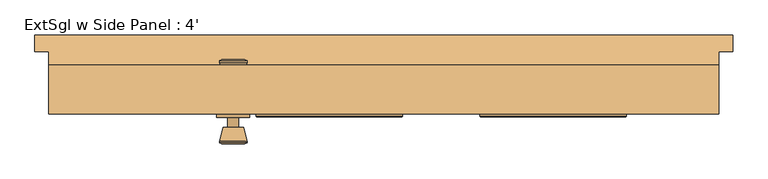
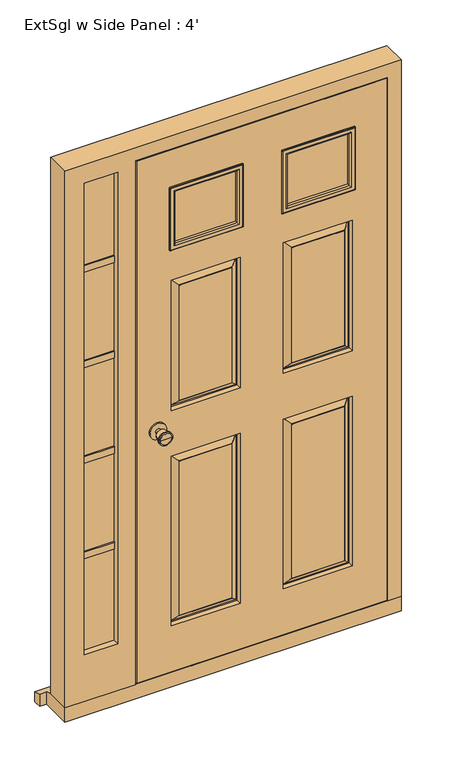
"""IFC4 building model written with IfcOpenShell, lengths in millimetres: door geometry, ExtSgl w Side Panel : 4'."""

from ifc_helpers import new_model, si_unit, point, frame, frame_2d, origin, place, context, project, spatial, polyline, circle_curve, ellipse_curve, trimmed, segment, composite_curve, outline, extrude, faceted_brep, source, transform, mapped, element, save
from ifc_brep_helpers import plane_surface, cylinder_surface, revolved_surface, advanced_brep


def extsgl_w_side_panel_4_ddded634(model_context):
    return source(origin(), model_context, "Body", "SolidModel", [
        advanced_brep(
        [(-493.3, -5.7, 1000.0), (-483.3, -5.7, 1000.0), (-503.3, -5.7, 1000.0), (-472.8241324, -54.7, 1000.0), (-493.3, -54.7, 1000.0), (-513.7758676, -54.7, 1000.0), (-468.3, -52.8721319, 1000.0), (-518.3, -52.8721319, 1000.0), (-468.3, -49.4084537, 1000.0), (-518.3, -49.4084537, 1000.0), (-474.663764, -24.7, 1000.0), (-511.936236, -24.7, 1000.0), (-483.3, -24.7, 1000.0), (-503.3, -24.7, 1000.0)],
        [
            (0, 1),
            (1, 2, circle_curve(frame((-493.3, -5.7, 1000.0), z_axis=(0.0, 1.0, 0.0), x_axis=(-1.0, 0.0, 0.0)), 10.0)),
            (2, 0),
            (2, 1, circle_curve(frame((-493.3, -5.7, 1000.0), z_axis=(0.0, 1.0, 0.0), x_axis=(-1.0, 0.0, 0.0)), 10.0)),
            (3, 4),
            (4, 5),
            (5, 3, circle_curve(frame((-493.3, -54.7, 1000.0), z_axis=(0.0, -1.0, 0.0), x_axis=(-1.0, 0.0, 0.0)), 20.4758676)),
            (3, 5, circle_curve(frame((-493.3, -54.7, 1000.0), z_axis=(0.0, -1.0, 0.0), x_axis=(-1.0, 0.0, 0.0)), 20.4758676)),
            (6, 3),
            (5, 7),
            (7, 6, circle_curve(frame((-493.3, -52.8721319, 1000.0), z_axis=(0.0, -1.0, 0.0), x_axis=(-1.0, 0.0, 0.0)), 25.0)),
            (6, 7, circle_curve(frame((-493.3, -52.8721319, 1000.0), z_axis=(0.0, -1.0, 0.0), x_axis=(-1.0, 0.0, 0.0)), 25.0)),
            (8, 6),
            (7, 9),
            (9, 8, circle_curve(frame((-493.3, -49.4084537, 1000.0), z_axis=(0.0, -1.0, 0.0), x_axis=(-1.0, 0.0, 0.0)), 25.0)),
            (8, 9, circle_curve(frame((-493.3, -49.4084537, 1000.0), z_axis=(0.0, -1.0, 0.0), x_axis=(-1.0, 0.0, 0.0)), 25.0)),
            (10, 8),
            (9, 11),
            (11, 10, circle_curve(frame((-493.3, -24.7, 1000.0), z_axis=(0.0, -1.0, 0.0), x_axis=(-1.0, 0.0, 0.0)), 18.636236)),
            (10, 11, circle_curve(frame((-493.3, -24.7, 1000.0), z_axis=(0.0, -1.0, 0.0), x_axis=(-1.0, 0.0, 0.0)), 18.636236)),
            (12, 10),
            (11, 13),
            (13, 12, circle_curve(frame((-493.3, -24.7, 1000.0), z_axis=(0.0, -1.0, 0.0), x_axis=(-1.0, 0.0, 0.0)), 10.0)),
            (12, 13, circle_curve(frame((-493.3, -24.7, 1000.0), z_axis=(0.0, -1.0, 0.0), x_axis=(-1.0, 0.0, 0.0)), 10.0)),
            (1, 12),
            (13, 2),
        ],
        [
            plane_surface(frame((-493.3, -5.7, 1000.0), z_axis=(0.0, 1.0, 0.0), x_axis=(-1.0, 0.0, 0.0))),
            plane_surface(frame((-493.3, -54.7, 1000.0), z_axis=(0.0, -1.0, 0.0), x_axis=(-1.0, 0.0, 0.0))),
            revolved_surface(polyline([(-513.7758676, -54.7, 1000.0), (-518.3, -52.8721319, 1000.0)]), (-493.3, -5.7, 1000.0), (0.0, 1.0, 0.0)),
            cylinder_surface(frame((-493.3, -5.7, 1000.0), z_axis=(0.0, 1.0, 0.0), x_axis=(-1.0, 0.0, 0.0)), 25.0),
            revolved_surface(polyline([(-518.3, -49.4084537, 1000.0), (-511.936236, -24.7, 1000.0)]), (-493.3, -5.7, 1000.0), (0.0, 1.0, 0.0)),
            plane_surface(frame((-493.3, -24.7, 1000.0), z_axis=(0.0, 1.0, 0.0), x_axis=(-1.0, 0.0, 0.0))),
            cylinder_surface(frame((-493.3, -5.7, 1000.0), z_axis=(0.0, 1.0, 0.0), x_axis=(-1.0, 0.0, 0.0)), 10.0),
        ],
        [
            (0, [[1, 2, 3]]),
            (0, [[-3, 4, -1]]),
            (1, [[5, 6, 7]]),
            (1, [[-6, -5, 8]]),
            (2, [[9, -7, 10, 11]]),
            (2, [[-10, -8, -9, 12]]),
            (3, [[13, -11, 14, 15]]),
            (3, [[-14, -12, -13, 16]]),
            (4, [[17, -15, 18, 19]]),
            (4, [[-18, -16, -17, 20]]),
            (5, [[21, -19, 22, 23]]),
            (5, [[-22, -20, -21, 24]]),
            (6, [[25, -23, 26, -2]]),
            (6, [[-26, -24, -25, -4]]),
        ],
    ),
        extrude(outline(composite_curve([segment(trimmed(circle_curve(frame_2d((1000.0, -493.3)), 30.0), [point((1000.0, -523.3))], [point((1000.0, -463.3))], False, "CARTESIAN"), True, "CONTINUOUS"), segment(trimmed(circle_curve(frame_2d((1000.0, -493.3)), 30.0), [point((1000.0, -463.3))], [point((1000.0, -523.3))], False, "CARTESIAN"), True, "CONTINUOUS")], self_intersect=False)), frame((0.0, -5.7, 0.0), z_axis=(0.0, 1.0, 0.0), x_axis=(0.0, 0.0, 1.0)), (0.0, 0.0, 1.0), 6.0),
        advanced_brep(
        [(-493.3, 50.3, 1000.0), (-503.3, 50.3, 1000.0), (-483.3, 50.3, 1000.0), (-472.8241324, 99.3, 1000.0), (-513.7758676, 99.3, 1000.0), (-493.3, 99.3, 1000.0), (-468.3, 97.4721319, 1000.0), (-518.3, 97.4721319, 1000.0), (-468.3, 94.0084537, 1000.0), (-518.3, 94.0084537, 1000.0), (-474.663764, 69.3, 1000.0), (-511.936236, 69.3, 1000.0), (-483.3, 69.3, 1000.0), (-503.3, 69.3, 1000.0)],
        [
            (0, 1),
            (1, 2, circle_curve(frame((-493.3, 50.3, 1000.0), z_axis=(0.0, -1.0, 0.0), x_axis=(-1.0, 0.0, 0.0)), 10.0)),
            (2, 0),
            (2, 1, circle_curve(frame((-493.3, 50.3, 1000.0), z_axis=(0.0, -1.0, 0.0), x_axis=(-1.0, 0.0, 0.0)), 10.0)),
            (3, 4, circle_curve(frame((-493.3, 99.3, 1000.0), z_axis=(0.0, 1.0, 0.0), x_axis=(-1.0, 0.0, 0.0)), 20.4758676)),
            (4, 5),
            (5, 3),
            (4, 3, circle_curve(frame((-493.3, 99.3, 1000.0), z_axis=(0.0, 1.0, 0.0), x_axis=(-1.0, 0.0, 0.0)), 20.4758676)),
            (6, 7, circle_curve(frame((-493.3, 97.4721319, 1000.0), z_axis=(0.0, 1.0, 0.0), x_axis=(-1.0, 0.0, 0.0)), 25.0)),
            (7, 4),
            (3, 6),
            (7, 6, circle_curve(frame((-493.3, 97.4721319, 1000.0), z_axis=(0.0, 1.0, 0.0), x_axis=(-1.0, 0.0, 0.0)), 25.0)),
            (8, 9, circle_curve(frame((-493.3, 94.0084537, 1000.0), z_axis=(0.0, 1.0, 0.0), x_axis=(-1.0, 0.0, 0.0)), 25.0)),
            (9, 7),
            (6, 8),
            (9, 8, circle_curve(frame((-493.3, 94.0084537, 1000.0), z_axis=(0.0, 1.0, 0.0), x_axis=(-1.0, 0.0, 0.0)), 25.0)),
            (10, 11, circle_curve(frame((-493.3, 69.3, 1000.0), z_axis=(0.0, 1.0, 0.0), x_axis=(-1.0, 0.0, 0.0)), 18.636236)),
            (11, 9),
            (8, 10),
            (11, 10, circle_curve(frame((-493.3, 69.3, 1000.0), z_axis=(0.0, 1.0, 0.0), x_axis=(-1.0, 0.0, 0.0)), 18.636236)),
            (12, 13, circle_curve(frame((-493.3, 69.3, 1000.0), z_axis=(0.0, 1.0, 0.0), x_axis=(-1.0, 0.0, 0.0)), 10.0)),
            (13, 11),
            (10, 12),
            (13, 12, circle_curve(frame((-493.3, 69.3, 1000.0), z_axis=(0.0, 1.0, 0.0), x_axis=(-1.0, 0.0, 0.0)), 10.0)),
            (1, 13),
            (12, 2),
        ],
        [
            plane_surface(frame((-493.3, 50.3, 1000.0), z_axis=(0.0, -1.0, 0.0), x_axis=(-1.0, 0.0, 0.0))),
            plane_surface(frame((-493.3, 99.3, 1000.0), z_axis=(0.0, 1.0, 0.0), x_axis=(-1.0, 0.0, 0.0))),
            revolved_surface(polyline([(-513.7758676, 99.3, 1000.0), (-518.3, 97.4721319, 1000.0)]), (-493.3, 50.3, 1000.0), (0.0, -1.0, 0.0)),
            cylinder_surface(frame((-493.3, 50.3, 1000.0), z_axis=(0.0, -1.0, 0.0), x_axis=(-1.0, 0.0, 0.0)), 25.0),
            revolved_surface(polyline([(-518.3, 94.0084537, 1000.0), (-511.936236, 69.3, 1000.0)]), (-493.3, 50.3, 1000.0), (0.0, -1.0, 0.0)),
            plane_surface(frame((-493.3, 69.3, 1000.0), z_axis=(0.0, -1.0, 0.0), x_axis=(-1.0, 0.0, 0.0))),
            cylinder_surface(frame((-493.3, 50.3, 1000.0), z_axis=(0.0, -1.0, 0.0), x_axis=(-1.0, 0.0, 0.0)), 10.0),
        ],
        [
            (0, [[1, 2, 3]]),
            (0, [[-3, 4, -1]]),
            (1, [[5, 6, 7]]),
            (1, [[8, -7, -6]]),
            (2, [[9, 10, -5, 11]]),
            (2, [[12, -11, -8, -10]]),
            (3, [[13, 14, -9, 15]]),
            (3, [[16, -15, -12, -14]]),
            (4, [[17, 18, -13, 19]]),
            (4, [[20, -19, -16, -18]]),
            (5, [[21, 22, -17, 23]]),
            (5, [[24, -23, -20, -22]]),
            (6, [[-2, 25, -21, 26]]),
            (6, [[-4, -26, -24, -25]]),
        ],
    ),
        extrude(outline(composite_curve([segment(trimmed(circle_curve(frame_2d((1000.0, -493.3)), 30.0), [point((1000.0, -523.3))], [point((1000.0, -463.3))], False, "CARTESIAN"), True, "CONTINUOUS"), segment(trimmed(circle_curve(frame_2d((1000.0, -493.3)), 30.0), [point((1000.0, -463.3))], [point((1000.0, -523.3))], False, "CARTESIAN"), True, "CONTINUOUS")], self_intersect=False)), frame((0.0, 44.3, 0.0), z_axis=(0.0, 1.0, 0.0), x_axis=(0.0, 0.0, 1.0)), (0.0, 0.0, 1.0), 6.0),
        faceted_brep([(319.7, 89.3, 54.5), (390.2, 89.3, 54.5), (390.2, 0.3, 54.5), (341.7, 0.3, 54.5), (341.7, 47.3, 54.5), (319.7, 47.3, 54.5), (319.7, 89.3, 2039.5), (-551.3, 89.3, 2039.5), (-551.3, 89.3, 54.5), (-829.0, 89.3, 54.5), (-829.0, 89.3, 2110.0), (390.2, 89.3, 2110.0), (-637.3, 89.3, 2039.5), (-758.5, 89.3, 2039.5), (-758.5, 89.3, 233.5), (-637.3, 89.3, 233.5), (390.2, 0.3, 2110.0), (-829.0, 0.3, 2110.0), (-829.0, 0.3, 54.5), (-573.3, 0.3, 54.5), (-573.3, 0.3, 2061.5), (341.7, 0.3, 2061.5), (-637.3, 0.3, 233.5), (-758.5, 0.3, 233.5), (-758.5, 0.3, 2039.5), (-637.3, 0.3, 2039.5), (341.7, 47.3, 2061.5), (-573.3, 47.3, 2061.5), (-573.3, 47.3, 54.5), (-551.3, 47.3, 54.5), (-551.3, 47.3, 2039.5), (319.7, 47.3, 2039.5), (-615.3, 47.3, 2061.5), (-780.5, 47.3, 2061.5), (-780.5, 47.3, 218.5), (-615.3, 47.3, 218.5), (-758.5, 47.3, 2039.5), (-637.3, 47.3, 2039.5), (-637.3, 47.3, 233.5), (-758.5, 47.3, 233.5), (-637.3, 23.3, 233.5), (-758.5, 23.3, 233.5), (-758.5, 23.3, 2039.5), (-637.3, 23.3, 2039.5), (-780.5, 23.3, 2061.5), (-780.5, 23.3, 218.5), (-615.3, 23.3, 218.5), (-615.3, 23.3, 2061.5)], [[[0, 1, 2, 3, 4, 5]], [[1, 0, 6, 7, 8, 9, 10, 11], [12, 13, 14, 15]], [[2, 1, 11, 16]], [[3, 2, 16, 17, 18, 19, 20, 21], [22, 23, 24, 25]], [[4, 3, 21, 26]], [[5, 4, 26, 27, 28, 29, 30, 31]], [[32, 33, 34, 35], [36, 37, 38, 39]], [[0, 5, 31, 6]], [[29, 8, 7, 30]], [[18, 9, 8, 29, 28, 19]], [[10, 9, 18, 17]], [[13, 36, 39, 14]], [[39, 38, 15, 14]], [[37, 12, 15, 38]], [[23, 22, 40, 41]], [[24, 23, 41, 42]], [[22, 25, 43, 40]], [[19, 28, 27, 20]], [[44, 45, 34, 33]], [[45, 46, 35, 34]], [[46, 47, 32, 35]], [[46, 45, 44, 47], [41, 40, 43, 42]], [[11, 10, 17, 16]], [[26, 21, 20, 27]], [[33, 32, 47, 44]], [[6, 31, 30, 7]], [[36, 13, 12, 37]], [[25, 24, 42, 43]]]),
        faceted_brep([(338.7, 0.3, 58.5), (338.7, 0.3, 2058.5), (-568.3, 0.3, 2058.5), (-568.3, 0.3, 58.5), (-36.3, 0.3, 1683.5), (-36.3, 0.3, 1908.5), (213.7, 0.3, 1908.5), (213.7, 0.3, 1683.5), (-443.3, 0.3, 1683.5), (-443.3, 0.3, 1908.5), (-193.3, 0.3, 1908.5), (-193.3, 0.3, 1683.5), (-193.3, 0.3, 883.5), (-193.3, 0.3, 233.5), (-443.3, 0.3, 233.5), (-443.3, 0.3, 883.5), (213.7, 0.3, 883.5), (213.7, 0.3, 233.5), (-36.3, 0.3, 233.5), (-36.3, 0.3, 883.5), (-193.3, 0.3, 1558.5), (-193.3, 0.3, 1058.5), (-443.3, 0.3, 1058.5), (-443.3, 0.3, 1558.5), (213.7, 0.3, 1558.5), (213.7, 0.3, 1058.5), (-36.3, 0.3, 1058.5), (-36.3, 0.3, 1558.5), (-223.3, 0.3, 263.5), (-223.3, 0.3, 853.5), (-413.3, 0.3, 853.5), (-413.3, 0.3, 263.5), (183.7, 0.3, 263.5), (183.7, 0.3, 853.5), (-6.3, 0.3, 853.5), (-6.3, 0.3, 263.5), (-223.3, 0.3, 1088.5), (-223.3, 0.3, 1528.5), (-413.3, 0.3, 1528.5), (-413.3, 0.3, 1088.5), (183.7, 0.3, 1088.5), (183.7, 0.3, 1528.5), (-6.3, 0.3, 1528.5), (-6.3, 0.3, 1088.5), (338.7, 44.3, 58.5), (-568.3, 44.3, 58.5), (-568.3, 44.3, 2058.5), (338.7, 44.3, 2058.5), (-36.3, 44.3, 1683.5), (213.7, 44.3, 1683.5), (213.7, 44.3, 1908.5), (-36.3, 44.3, 1908.5), (-443.3, 44.3, 1683.5), (-193.3, 44.3, 1683.5), (-193.3, 44.3, 1908.5), (-443.3, 44.3, 1908.5), (-36.3, 44.3, 883.5), (-36.3, 44.3, 233.5), (213.7, 44.3, 233.5), (213.7, 44.3, 883.5), (-443.3, 44.3, 883.5), (-443.3, 44.3, 233.5), (-193.3, 44.3, 233.5), (-193.3, 44.3, 883.5), (-36.3, 44.3, 1558.5), (-36.3, 44.3, 1058.5), (213.7, 44.3, 1058.5), (213.7, 44.3, 1558.5), (-443.3, 44.3, 1558.5), (-443.3, 44.3, 1058.5), (-193.3, 44.3, 1058.5), (-193.3, 44.3, 1558.5), (-6.3, 44.3, 263.5), (-6.3, 44.3, 853.5), (183.7, 44.3, 853.5), (183.7, 44.3, 263.5), (-413.3, 44.3, 263.5), (-413.3, 44.3, 853.5), (-223.3, 44.3, 853.5), (-223.3, 44.3, 263.5), (-6.3, 44.3, 1088.5), (-6.3, 44.3, 1528.5), (183.7, 44.3, 1528.5), (183.7, 44.3, 1088.5), (-413.3, 44.3, 1088.5), (-413.3, 44.3, 1528.5), (-223.3, 44.3, 1528.5), (-223.3, 44.3, 1088.5), (-33.3, 29.3, 880.5), (-33.3, 29.3, 236.5), (-8.3, 43.3, 855.5), (-8.3, 43.3, 261.5), (-28.3, 29.3, 241.5), (-28.3, 29.3, 875.5), (-6.3, 43.3, 263.5), (-6.3, 43.3, 853.5), (210.7, 29.3, 236.5), (185.7, 43.3, 261.5), (205.7, 29.3, 241.5), (183.7, 43.3, 263.5), (210.7, 29.3, 880.5), (185.7, 43.3, 855.5), (205.7, 29.3, 875.5), (183.7, 43.3, 853.5), (-440.3, 29.3, 880.5), (-440.3, 29.3, 236.5), (-415.3, 43.3, 855.5), (-415.3, 43.3, 261.5), (-435.3, 29.3, 241.5), (-435.3, 29.3, 875.5), (-413.3, 43.3, 263.5), (-413.3, 43.3, 853.5), (-196.3, 29.3, 236.5), (-221.3, 43.3, 261.5), (-201.3, 29.3, 241.5), (-223.3, 43.3, 263.5), (-196.3, 29.3, 880.5), (-221.3, 43.3, 855.5), (-201.3, 29.3, 875.5), (-223.3, 43.3, 853.5), (-223.3, 1.3, 263.5), (-223.3, 1.3, 853.5), (-201.3, 15.3, 241.5), (-201.3, 15.3, 875.5), (-221.3, 1.3, 855.5), (-221.3, 1.3, 261.5), (-196.3, 15.3, 880.5), (-196.3, 15.3, 236.5), (-413.3, 1.3, 853.5), (-435.3, 15.3, 875.5), (-415.3, 1.3, 855.5), (-440.3, 15.3, 880.5), (-413.3, 1.3, 263.5), (-435.3, 15.3, 241.5), (-415.3, 1.3, 261.5), (-440.3, 15.3, 236.5), (210.7, 15.3, 880.5), (210.7, 15.3, 236.5), (185.7, 1.3, 855.5), (185.7, 1.3, 261.5), (205.7, 15.3, 241.5), (205.7, 15.3, 875.5), (183.7, 1.3, 263.5), (183.7, 1.3, 853.5), (-33.3, 15.3, 236.5), (-8.3, 1.3, 261.5), (-28.3, 15.3, 241.5), (-6.3, 1.3, 263.5), (-33.3, 15.3, 880.5), (-8.3, 1.3, 855.5), (-28.3, 15.3, 875.5), (-6.3, 1.3, 853.5), (-6.3, 43.3, 1088.5), (-6.3, 43.3, 1528.5), (-28.3, 29.3, 1066.5), (-28.3, 29.3, 1550.5), (-8.3, 43.3, 1530.5), (-8.3, 43.3, 1086.5), (-33.3, 29.3, 1555.5), (-33.3, 29.3, 1061.5), (183.7, 43.3, 1528.5), (205.7, 29.3, 1550.5), (185.7, 43.3, 1530.5), (210.7, 29.3, 1555.5), (183.7, 43.3, 1088.5), (205.7, 29.3, 1066.5), (185.7, 43.3, 1086.5), (210.7, 29.3, 1061.5), (-413.3, 43.3, 1088.5), (-413.3, 43.3, 1528.5), (-435.3, 29.3, 1066.5), (-435.3, 29.3, 1550.5), (-415.3, 43.3, 1530.5), (-415.3, 43.3, 1086.5), (-440.3, 29.3, 1555.5), (-440.3, 29.3, 1061.5), (-223.3, 43.3, 1528.5), (-201.3, 29.3, 1550.5), (-221.3, 43.3, 1530.5), (-196.3, 29.3, 1555.5), (-223.3, 43.3, 1088.5), (-201.3, 29.3, 1066.5), (-221.3, 43.3, 1086.5), (-196.3, 29.3, 1061.5), (-223.3, 1.3, 1088.5), (-223.3, 1.3, 1528.5), (-201.3, 15.3, 1066.5), (-201.3, 15.3, 1550.5), (-221.3, 1.3, 1530.5), (-221.3, 1.3, 1086.5), (-196.3, 15.3, 1555.5), (-196.3, 15.3, 1061.5), (-413.3, 1.3, 1528.5), (-435.3, 15.3, 1550.5), (-415.3, 1.3, 1530.5), (-440.3, 15.3, 1555.5), (-413.3, 1.3, 1088.5), (-435.3, 15.3, 1066.5), (-415.3, 1.3, 1086.5), (-440.3, 15.3, 1061.5), (210.7, 15.3, 1555.5), (210.7, 15.3, 1061.5), (185.7, 1.3, 1530.5), (185.7, 1.3, 1086.5), (205.7, 15.3, 1066.5), (205.7, 15.3, 1550.5), (183.7, 1.3, 1088.5), (183.7, 1.3, 1528.5), (-33.3, 15.3, 1061.5), (-8.3, 1.3, 1086.5), (-28.3, 15.3, 1066.5), (-6.3, 1.3, 1088.5), (-33.3, 15.3, 1555.5), (-8.3, 1.3, 1530.5), (-28.3, 15.3, 1550.5), (-6.3, 1.3, 1528.5)], [[[0, 1, 2, 3], [4, 5, 6, 7], [8, 9, 10, 11], [12, 13, 14, 15], [16, 17, 18, 19], [20, 21, 22, 23], [24, 25, 26, 27]], [[28, 29, 30, 31]], [[32, 33, 34, 35]], [[36, 37, 38, 39]], [[40, 41, 42, 43]], [[44, 45, 46, 47], [48, 49, 50, 51], [52, 53, 54, 55], [56, 57, 58, 59], [60, 61, 62, 63], [64, 65, 66, 67], [68, 69, 70, 71]], [[72, 73, 74, 75]], [[76, 77, 78, 79]], [[80, 81, 82, 83]], [[84, 85, 86, 87]], [[1, 0, 44, 47]], [[2, 1, 47, 46]], [[3, 2, 46, 45]], [[0, 3, 45, 44]], [[5, 4, 48, 51]], [[6, 5, 51, 50]], [[7, 6, 50, 49]], [[4, 7, 49, 48]], [[9, 8, 52, 55]], [[10, 9, 55, 54]], [[11, 10, 54, 53]], [[8, 11, 53, 52]], [[88, 89, 57, 56]], [[90, 91, 92, 93]], [[72, 94, 95, 73]], [[57, 89, 96, 58]], [[92, 91, 97, 98]], [[94, 72, 75, 99]], [[58, 96, 100, 59]], [[98, 97, 101, 102]], [[99, 75, 74, 103]], [[88, 56, 59, 100]], [[89, 88, 100, 96], [93, 92, 98, 102]], [[90, 93, 102, 101]], [[91, 90, 101, 97], [95, 94, 99, 103]], [[73, 95, 103, 74]], [[104, 105, 61, 60]], [[106, 107, 108, 109]], [[76, 110, 111, 77]], [[61, 105, 112, 62]], [[108, 107, 113, 114]], [[110, 76, 79, 115]], [[62, 112, 116, 63]], [[114, 113, 117, 118]], [[115, 79, 78, 119]], [[104, 60, 63, 116]], [[105, 104, 116, 112], [109, 108, 114, 118]], [[106, 109, 118, 117]], [[107, 106, 117, 113], [111, 110, 115, 119]], [[77, 111, 119, 78]], [[120, 121, 29, 28]], [[122, 123, 124, 125]], [[12, 126, 127, 13]], [[29, 121, 128, 30]], [[124, 123, 129, 130]], [[126, 12, 15, 131]], [[30, 128, 132, 31]], [[130, 129, 133, 134]], [[131, 15, 14, 135]], [[120, 28, 31, 132]], [[125, 124, 130, 134], [121, 120, 132, 128]], [[122, 125, 134, 133]], [[127, 126, 131, 135], [123, 122, 133, 129]], [[13, 127, 135, 14]], [[136, 137, 17, 16]], [[138, 139, 140, 141]], [[32, 142, 143, 33]], [[17, 137, 144, 18]], [[140, 139, 145, 146]], [[142, 32, 35, 147]], [[18, 144, 148, 19]], [[146, 145, 149, 150]], [[147, 35, 34, 151]], [[136, 16, 19, 148]], [[137, 136, 148, 144], [141, 140, 146, 150]], [[138, 141, 150, 149]], [[139, 138, 149, 145], [143, 142, 147, 151]], [[33, 143, 151, 34]], [[152, 153, 81, 80]], [[154, 155, 156, 157]], [[64, 158, 159, 65]], [[81, 153, 160, 82]], [[156, 155, 161, 162]], [[158, 64, 67, 163]], [[82, 160, 164, 83]], [[162, 161, 165, 166]], [[163, 67, 66, 167]], [[152, 80, 83, 164]], [[157, 156, 162, 166], [153, 152, 164, 160]], [[154, 157, 166, 165]], [[159, 158, 163, 167], [155, 154, 165, 161]], [[65, 159, 167, 66]], [[168, 169, 85, 84]], [[170, 171, 172, 173]], [[68, 174, 175, 69]], [[85, 169, 176, 86]], [[172, 171, 177, 178]], [[174, 68, 71, 179]], [[86, 176, 180, 87]], [[178, 177, 181, 182]], [[179, 71, 70, 183]], [[168, 84, 87, 180]], [[173, 172, 178, 182], [169, 168, 180, 176]], [[170, 173, 182, 181]], [[175, 174, 179, 183], [171, 170, 181, 177]], [[69, 175, 183, 70]], [[184, 185, 37, 36]], [[186, 187, 188, 189]], [[20, 190, 191, 21]], [[37, 185, 192, 38]], [[188, 187, 193, 194]], [[190, 20, 23, 195]], [[38, 192, 196, 39]], [[194, 193, 197, 198]], [[195, 23, 22, 199]], [[184, 36, 39, 196]], [[189, 188, 194, 198], [185, 184, 196, 192]], [[186, 189, 198, 197]], [[191, 190, 195, 199], [187, 186, 197, 193]], [[21, 191, 199, 22]], [[200, 201, 25, 24]], [[202, 203, 204, 205]], [[40, 206, 207, 41]], [[25, 201, 208, 26]], [[204, 203, 209, 210]], [[206, 40, 43, 211]], [[26, 208, 212, 27]], [[210, 209, 213, 214]], [[211, 43, 42, 215]], [[200, 24, 27, 212]], [[201, 200, 212, 208], [205, 204, 210, 214]], [[202, 205, 214, 213]], [[203, 202, 213, 209], [207, 206, 211, 215]], [[41, 207, 215, 42]]]),
        faceted_brep([(415.2, 144.3, 0.0), (415.2, 144.3, 38.5947221), (415.2, 114.3, 47.2703282), (415.2, 114.3, 0.0), (-854.0, 144.3, 38.5947221), (-854.0, 144.3, 0.0), (-854.0, 114.3, 0.0), (-854.0, 114.3, 47.2703282), (390.2, 114.3, 0.0), (390.2, 0.3, 0.0), (-829.0, 0.3, 0.0), (-829.0, 114.3, 0.0), (-829.0, 114.3, 47.2703282), (-829.0, 89.3, 54.5), (390.2, 89.3, 54.5), (390.2, 114.3, 47.2703282), (-829.0, 0.3, 54.5), (390.2, 0.3, 54.5)], [[[0, 1, 2, 3]], [[4, 5, 6, 7]], [[5, 0, 3, 8, 9, 10, 11, 6]], [[1, 0, 5, 4]], [[1, 4, 7, 12, 13, 14, 15, 2]], [[13, 16, 17, 14]], [[16, 10, 9, 17]], [[12, 11, 10, 16, 13]], [[11, 12, 7, 6]], [[8, 15, 14, 17, 9]], [[15, 8, 3, 2]]]),
        extrude(outline(polyline([(213.7, 10.3), (-36.3, 10.3), (-36.3, 34.3), (213.7, 34.3), (213.7, 10.3)])), frame((0.0, 0.0, 1683.5), z_axis=(0.0, 0.0, 1.0), x_axis=(1.0, 0.0, 0.0)), (0.0, 0.0, 1.0), 225.0),
        extrude(outline(polyline([(-193.3, 10.3), (-443.3, 10.3), (-443.3, 34.3), (-193.3, 34.3), (-193.3, 10.3)])), frame((0.0, 0.0, 1683.5), z_axis=(0.0, 0.0, 1.0), x_axis=(1.0, 0.0, 0.0)), (0.0, 0.0, 1.0), 225.0),
        advanced_brep(
        [(-44.3, 48.3, 1675.5), (-44.3, 44.3, 1675.5), (-44.3, 44.3, 1916.5), (-44.3, 48.3, 1916.5), (-42.3, 50.3, 1677.5), (-42.3, 50.3, 1914.5), (-24.3, 45.3, 1695.5), (-29.3, 50.3, 1690.5), (-29.3, 50.3, 1901.5), (-24.3, 45.3, 1896.5), (-24.3, 34.3, 1695.5), (-24.3, 34.3, 1896.5), (-36.3, 44.3, 1683.5), (-36.3, 34.3, 1683.5), (-36.3, 34.3, 1908.5), (-36.3, 44.3, 1908.5), (221.7, 44.3, 1916.5), (221.7, 48.3, 1916.5), (219.7, 50.3, 1914.5), (206.7, 50.3, 1901.5), (201.7, 45.3, 1896.5), (201.7, 34.3, 1896.5), (213.7, 34.3, 1908.5), (213.7, 44.3, 1908.5), (221.7, 44.3, 1675.5), (221.7, 48.3, 1675.5), (219.7, 50.3, 1677.5), (206.7, 50.3, 1690.5), (201.7, 45.3, 1695.5), (201.7, 34.3, 1695.5), (213.7, 34.3, 1683.5), (213.7, 44.3, 1683.5)],
        [
            (0, 1),
            (1, 2),
            (2, 3),
            (3, 0),
            (4, 0, ellipse_curve(frame((-42.3, 48.3, 1677.5), z_axis=(-0.7071067811865475, 0.0, 0.7071067811865475), x_axis=(-0.7071067811865474, 0.0, -0.7071067811865476)), 2.8284271, 2.0)),
            (3, 5, ellipse_curve(frame((-42.3, 48.3, 1914.5), z_axis=(-0.7071067811865475, 0.0, -0.7071067811865475), x_axis=(0.7071067811865474, 0.0, -0.7071067811865476)), 2.8284271, 2.0)),
            (5, 4),
            (6, 7, ellipse_curve(frame((-29.3, 45.3, 1690.5), z_axis=(-0.7071067811865475, 0.0, 0.7071067811865475), x_axis=(-0.7071067811865474, 0.0, -0.7071067811865476)), 7.0710678, 5.0)),
            (7, 8),
            (8, 9, ellipse_curve(frame((-29.3, 45.3, 1901.5), z_axis=(-0.7071067811865475, 0.0, -0.7071067811865475), x_axis=(0.7071067811865474, 0.0, -0.7071067811865476)), 7.0710678, 5.0)),
            (9, 6),
            (10, 6),
            (9, 11),
            (11, 10),
            (12, 13),
            (13, 14),
            (14, 15),
            (15, 12),
            (2, 16),
            (16, 17),
            (17, 3),
            (17, 18, ellipse_curve(frame((219.7, 48.3, 1914.5), z_axis=(-0.7071067811865475, 0.0, 0.7071067811865475), x_axis=(-0.7071067811865476, 0.0, -0.7071067811865474)), 2.8284271, 2.0)),
            (18, 5),
            (8, 19),
            (19, 20, ellipse_curve(frame((206.7, 45.3, 1901.5), z_axis=(-0.7071067811865475, 0.0, 0.7071067811865475), x_axis=(-0.7071067811865476, 0.0, -0.7071067811865474)), 7.0710678, 5.0)),
            (20, 9),
            (20, 21),
            (21, 11),
            (14, 22),
            (22, 23),
            (23, 15),
            (16, 24),
            (24, 25),
            (25, 17),
            (25, 26, ellipse_curve(frame((219.7, 48.3, 1677.5), z_axis=(0.7071067811865475, 0.0, 0.7071067811865475), x_axis=(-0.7071067811865474, 0.0, 0.7071067811865476)), 2.8284271, 2.0)),
            (26, 18),
            (19, 27),
            (27, 28, ellipse_curve(frame((206.7, 45.3, 1690.5), z_axis=(0.7071067811865475, 0.0, 0.7071067811865475), x_axis=(-0.7071067811865474, 0.0, 0.7071067811865476)), 7.0710678, 5.0)),
            (28, 20),
            (28, 29),
            (29, 21),
            (22, 30),
            (30, 31),
            (31, 23),
            (24, 1),
            (0, 25),
            (4, 26),
            (7, 27),
            (6, 28),
            (10, 29),
            (13, 30),
            (12, 31),
        ],
        [
            plane_surface(frame((-44.3, 44.3, 1675.5), z_axis=(-1.0, 0.0, 0.0), x_axis=(0.0, 0.0, 1.0))),
            cylinder_surface(frame((-42.3, 48.3, 1683.5), z_axis=(0.0, 0.0, -1.0), x_axis=(-1.0, 0.0, 0.0)), 2.0),
            cylinder_surface(frame((-29.3, 45.3, 1683.5), z_axis=(0.0, 0.0, -1.0), x_axis=(-1.0, 0.0, 0.0)), 5.0),
            plane_surface(frame((-24.3, 45.3, 1695.5), z_axis=(1.0, 0.0, 0.0), x_axis=(0.0, 0.0, 1.0))),
            plane_surface(frame((-36.3, 34.3, 1683.5), z_axis=(-1.0, 0.0, 0.0), x_axis=(0.0, 0.0, 1.0))),
            plane_surface(frame((-44.3, 44.3, 1916.5), z_axis=(0.0, 0.0, 1.0), x_axis=(1.0, 0.0, 0.0))),
            cylinder_surface(frame((-36.3, 48.3, 1914.5), z_axis=(-1.0, 0.0, 0.0), x_axis=(0.0, 0.0, 1.0)), 2.0),
            cylinder_surface(frame((-36.3, 45.3, 1901.5), z_axis=(-1.0, 0.0, 0.0), x_axis=(0.0, 0.0, 1.0)), 5.0),
            plane_surface(frame((-24.3, 45.3, 1896.5), z_axis=(0.0, 0.0, -1.0), x_axis=(1.0, 0.0, 0.0))),
            plane_surface(frame((-36.3, 34.3, 1908.5), z_axis=(0.0, 0.0, 1.0), x_axis=(1.0, 0.0, 0.0))),
            plane_surface(frame((221.7, 44.3, 1916.5), z_axis=(1.0, 0.0, 0.0), x_axis=(0.0, 0.0, -1.0))),
            cylinder_surface(frame((219.7, 48.3, 1908.5), z_axis=(0.0, 0.0, 1.0), x_axis=(1.0, 0.0, 0.0)), 2.0),
            cylinder_surface(frame((206.7, 45.3, 1908.5), z_axis=(0.0, 0.0, 1.0), x_axis=(1.0, 0.0, 0.0)), 5.0),
            plane_surface(frame((201.7, 45.3, 1896.5), z_axis=(-1.0, 0.0, 0.0), x_axis=(0.0, 0.0, -1.0))),
            plane_surface(frame((213.7, 34.3, 1908.5), z_axis=(1.0, 0.0, 0.0), x_axis=(0.0, 0.0, -1.0))),
            plane_surface(frame((221.7, 44.3, 1675.5), z_axis=(0.0, 0.0, -1.0), x_axis=(-1.0, 0.0, 0.0))),
            cylinder_surface(frame((213.7, 48.3, 1677.5), z_axis=(1.0, 0.0, 0.0), x_axis=(0.0, 0.0, -1.0)), 2.0),
            plane_surface(frame((219.7, 50.3, 1677.5), z_axis=(0.0, 1.0, 0.0), x_axis=(-1.0, 0.0, 0.0))),
            cylinder_surface(frame((213.7, 45.3, 1690.5), z_axis=(1.0, 0.0, 0.0), x_axis=(0.0, 0.0, -1.0)), 5.0),
            plane_surface(frame((201.7, 45.3, 1695.5), z_axis=(0.0, 0.0, 1.0), x_axis=(-1.0, 0.0, 0.0))),
            plane_surface(frame((201.7, 34.3, 1695.5), z_axis=(0.0, -1.0, 0.0), x_axis=(-1.0, 0.0, 0.0))),
            plane_surface(frame((213.7, 34.3, 1683.5), z_axis=(0.0, 0.0, -1.0), x_axis=(-1.0, 0.0, 0.0))),
            plane_surface(frame((213.7, 44.3, 1683.5), z_axis=(0.0, -1.0, 0.0), x_axis=(-1.0, 0.0, 0.0))),
        ],
        [
            (0, [[1, 2, 3, 4]]),
            (1, [[5, -4, 6, 7]]),
            (2, [[8, 9, 10, 11]]),
            (3, [[12, -11, 13, 14]]),
            (4, [[15, 16, 17, 18]]),
            (5, [[-3, 19, 20, 21]]),
            (6, [[-6, -21, 22, 23]]),
            (7, [[-10, 24, 25, 26]]),
            (8, [[-13, -26, 27, 28]]),
            (9, [[-17, 29, 30, 31]]),
            (10, [[-20, 32, 33, 34]]),
            (11, [[-22, -34, 35, 36]]),
            (12, [[-25, 37, 38, 39]]),
            (13, [[-27, -39, 40, 41]]),
            (14, [[-30, 42, 43, 44]]),
            (15, [[-33, 45, -1, 46]]),
            (16, [[-35, -46, -5, 47]]),
            (17, [[-23, -36, -47, -7], [48, -37, -24, -9]]),
            (18, [[-38, -48, -8, 49]]),
            (19, [[-40, -49, -12, 50]]),
            (20, [[51, -42, -29, -16], [-28, -41, -50, -14]]),
            (21, [[-43, -51, -15, 52]]),
            (22, [[-45, -32, -19, -2], [-31, -44, -52, -18]]),
        ],
    ),
        advanced_brep(
        [(-451.3, 48.3, 1675.5), (-451.3, 44.3, 1675.5), (-451.3, 44.3, 1916.5), (-451.3, 48.3, 1916.5), (-449.3, 50.3, 1677.5), (-449.3, 50.3, 1914.5), (-431.3, 45.3, 1695.5), (-436.3, 50.3, 1690.5), (-436.3, 50.3, 1901.5), (-431.3, 45.3, 1896.5), (-431.3, 34.3, 1695.5), (-431.3, 34.3, 1896.5), (-443.3, 44.3, 1683.5), (-443.3, 34.3, 1683.5), (-443.3, 34.3, 1908.5), (-443.3, 44.3, 1908.5), (-185.3, 44.3, 1916.5), (-185.3, 48.3, 1916.5), (-187.3, 50.3, 1914.5), (-200.3, 50.3, 1901.5), (-205.3, 45.3, 1896.5), (-205.3, 34.3, 1896.5), (-193.3, 34.3, 1908.5), (-193.3, 44.3, 1908.5), (-185.3, 44.3, 1675.5), (-185.3, 48.3, 1675.5), (-187.3, 50.3, 1677.5), (-200.3, 50.3, 1690.5), (-205.3, 45.3, 1695.5), (-205.3, 34.3, 1695.5), (-193.3, 34.3, 1683.5), (-193.3, 44.3, 1683.5)],
        [
            (0, 1),
            (1, 2),
            (2, 3),
            (3, 0),
            (4, 0, ellipse_curve(frame((-449.3, 48.3, 1677.5), z_axis=(-0.7071067811865475, 0.0, 0.7071067811865475), x_axis=(-0.7071067811865474, 0.0, -0.7071067811865476)), 2.8284271, 2.0)),
            (3, 5, ellipse_curve(frame((-449.3, 48.3, 1914.5), z_axis=(-0.7071067811865475, 0.0, -0.7071067811865475), x_axis=(0.7071067811865474, 0.0, -0.7071067811865476)), 2.8284271, 2.0)),
            (5, 4),
            (6, 7, ellipse_curve(frame((-436.3, 45.3, 1690.5), z_axis=(-0.7071067811865475, 0.0, 0.7071067811865475), x_axis=(-0.7071067811865474, 0.0, -0.7071067811865476)), 7.0710678, 5.0)),
            (7, 8),
            (8, 9, ellipse_curve(frame((-436.3, 45.3, 1901.5), z_axis=(-0.7071067811865475, 0.0, -0.7071067811865475), x_axis=(0.7071067811865474, 0.0, -0.7071067811865476)), 7.0710678, 5.0)),
            (9, 6),
            (10, 6),
            (9, 11),
            (11, 10),
            (12, 13),
            (13, 14),
            (14, 15),
            (15, 12),
            (2, 16),
            (16, 17),
            (17, 3),
            (17, 18, ellipse_curve(frame((-187.3, 48.3, 1914.5), z_axis=(-0.7071067811865475, 0.0, 0.7071067811865475), x_axis=(-0.7071067811865476, 0.0, -0.7071067811865474)), 2.8284271, 2.0)),
            (18, 5),
            (8, 19),
            (19, 20, ellipse_curve(frame((-200.3, 45.3, 1901.5), z_axis=(-0.7071067811865475, 0.0, 0.7071067811865475), x_axis=(-0.7071067811865476, 0.0, -0.7071067811865474)), 7.0710678, 5.0)),
            (20, 9),
            (20, 21),
            (21, 11),
            (14, 22),
            (22, 23),
            (23, 15),
            (16, 24),
            (24, 25),
            (25, 17),
            (25, 26, ellipse_curve(frame((-187.3, 48.3, 1677.5), z_axis=(0.7071067811865475, 0.0, 0.7071067811865475), x_axis=(-0.7071067811865474, 0.0, 0.7071067811865476)), 2.8284271, 2.0)),
            (26, 18),
            (19, 27),
            (27, 28, ellipse_curve(frame((-200.3, 45.3, 1690.5), z_axis=(0.7071067811865475, 0.0, 0.7071067811865475), x_axis=(-0.7071067811865474, 0.0, 0.7071067811865476)), 7.0710678, 5.0)),
            (28, 20),
            (28, 29),
            (29, 21),
            (22, 30),
            (30, 31),
            (31, 23),
            (24, 1),
            (0, 25),
            (4, 26),
            (7, 27),
            (6, 28),
            (10, 29),
            (13, 30),
            (12, 31),
        ],
        [
            plane_surface(frame((-451.3, 44.3, 1675.5), z_axis=(-1.0, 0.0, 0.0), x_axis=(0.0, 0.0, 1.0))),
            cylinder_surface(frame((-449.3, 48.3, 1683.5), z_axis=(0.0, 0.0, -1.0), x_axis=(-1.0, 0.0, 0.0)), 2.0),
            cylinder_surface(frame((-436.3, 45.3, 1683.5), z_axis=(0.0, 0.0, -1.0), x_axis=(-1.0, 0.0, 0.0)), 5.0),
            plane_surface(frame((-431.3, 45.3, 1695.5), z_axis=(1.0, 0.0, 0.0), x_axis=(0.0, 0.0, 1.0))),
            plane_surface(frame((-443.3, 34.3, 1683.5), z_axis=(-1.0, 0.0, 0.0), x_axis=(0.0, 0.0, 1.0))),
            plane_surface(frame((-451.3, 44.3, 1916.5), z_axis=(0.0, 0.0, 1.0), x_axis=(1.0, 0.0, 0.0))),
            cylinder_surface(frame((-443.3, 48.3, 1914.5), z_axis=(-1.0, 0.0, 0.0), x_axis=(0.0, 0.0, 1.0)), 2.0),
            cylinder_surface(frame((-443.3, 45.3, 1901.5), z_axis=(-1.0, 0.0, 0.0), x_axis=(0.0, 0.0, 1.0)), 5.0),
            plane_surface(frame((-431.3, 45.3, 1896.5), z_axis=(0.0, 0.0, -1.0), x_axis=(1.0, 0.0, 0.0))),
            plane_surface(frame((-443.3, 34.3, 1908.5), z_axis=(0.0, 0.0, 1.0), x_axis=(1.0, 0.0, 0.0))),
            plane_surface(frame((-185.3, 44.3, 1916.5), z_axis=(1.0, 0.0, 0.0), x_axis=(0.0, 0.0, -1.0))),
            cylinder_surface(frame((-187.3, 48.3, 1908.5), z_axis=(0.0, 0.0, 1.0), x_axis=(1.0, 0.0, 0.0)), 2.0),
            cylinder_surface(frame((-200.3, 45.3, 1908.5), z_axis=(0.0, 0.0, 1.0), x_axis=(1.0, 0.0, 0.0)), 5.0),
            plane_surface(frame((-205.3, 45.3, 1896.5), z_axis=(-1.0, 0.0, 0.0), x_axis=(0.0, 0.0, -1.0))),
            plane_surface(frame((-193.3, 34.3, 1908.5), z_axis=(1.0, 0.0, 0.0), x_axis=(0.0, 0.0, -1.0))),
            plane_surface(frame((-185.3, 44.3, 1675.5), z_axis=(0.0, 0.0, -1.0), x_axis=(-1.0, 0.0, 0.0))),
            cylinder_surface(frame((-193.3, 48.3, 1677.5), z_axis=(1.0, 0.0, 0.0), x_axis=(0.0, 0.0, -1.0)), 2.0),
            plane_surface(frame((-187.3, 50.3, 1677.5), z_axis=(0.0, 1.0, 0.0), x_axis=(-1.0, 0.0, 0.0))),
            cylinder_surface(frame((-193.3, 45.3, 1690.5), z_axis=(1.0, 0.0, 0.0), x_axis=(0.0, 0.0, -1.0)), 5.0),
            plane_surface(frame((-205.3, 45.3, 1695.5), z_axis=(0.0, 0.0, 1.0), x_axis=(-1.0, 0.0, 0.0))),
            plane_surface(frame((-205.3, 34.3, 1695.5), z_axis=(0.0, -1.0, 0.0), x_axis=(-1.0, 0.0, 0.0))),
            plane_surface(frame((-193.3, 34.3, 1683.5), z_axis=(0.0, 0.0, -1.0), x_axis=(-1.0, 0.0, 0.0))),
            plane_surface(frame((-193.3, 44.3, 1683.5), z_axis=(0.0, -1.0, 0.0), x_axis=(-1.0, 0.0, 0.0))),
        ],
        [
            (0, [[1, 2, 3, 4]]),
            (1, [[5, -4, 6, 7]]),
            (2, [[8, 9, 10, 11]]),
            (3, [[12, -11, 13, 14]]),
            (4, [[15, 16, 17, 18]]),
            (5, [[-3, 19, 20, 21]]),
            (6, [[-6, -21, 22, 23]]),
            (7, [[-10, 24, 25, 26]]),
            (8, [[-13, -26, 27, 28]]),
            (9, [[-17, 29, 30, 31]]),
            (10, [[-20, 32, 33, 34]]),
            (11, [[-22, -34, 35, 36]]),
            (12, [[-25, 37, 38, 39]]),
            (13, [[-27, -39, 40, 41]]),
            (14, [[-30, 42, 43, 44]]),
            (15, [[-33, 45, -1, 46]]),
            (16, [[-35, -46, -5, 47]]),
            (17, [[-23, -36, -47, -7], [48, -37, -24, -9]]),
            (18, [[-38, -48, -8, 49]]),
            (19, [[-40, -49, -12, 50]]),
            (20, [[51, -42, -29, -16], [-28, -41, -50, -14]]),
            (21, [[-43, -51, -15, 52]]),
            (22, [[-45, -32, -19, -2], [-31, -44, -52, -18]]),
        ],
    ),
        advanced_brep(
        [(-185.3, -3.7, 1675.5), (-185.3, 0.3, 1675.5), (-185.3, 0.3, 1916.5), (-185.3, -3.7, 1916.5), (-187.3, -5.7, 1677.5), (-187.3, -5.7, 1914.5), (-205.3, -0.7, 1695.5), (-200.3, -5.7, 1690.5), (-200.3, -5.7, 1901.5), (-205.3, -0.7, 1896.5), (-205.3, 10.3, 1695.5), (-205.3, 10.3, 1896.5), (-193.3, 0.3, 1683.5), (-193.3, 10.3, 1683.5), (-193.3, 10.3, 1908.5), (-193.3, 0.3, 1908.5), (-451.3, 0.3, 1916.5), (-451.3, -3.7, 1916.5), (-449.3, -5.7, 1914.5), (-436.3, -5.7, 1901.5), (-431.3, -0.7, 1896.5), (-431.3, 10.3, 1896.5), (-443.3, 10.3, 1908.5), (-443.3, 0.3, 1908.5), (-451.3, 0.3, 1675.5), (-451.3, -3.7, 1675.5), (-449.3, -5.7, 1677.5), (-436.3, -5.7, 1690.5), (-431.3, -0.7, 1695.5), (-431.3, 10.3, 1695.5), (-443.3, 10.3, 1683.5), (-443.3, 0.3, 1683.5)],
        [
            (0, 1),
            (1, 2),
            (2, 3),
            (3, 0),
            (4, 0, ellipse_curve(frame((-187.3, -3.7, 1677.5), z_axis=(0.7071067811865475, 0.0, 0.7071067811865475), x_axis=(0.7071067811865474, 0.0, -0.7071067811865476)), 2.8284271, 2.0)),
            (3, 5, ellipse_curve(frame((-187.3, -3.7, 1914.5), z_axis=(0.7071067811865475, 0.0, -0.7071067811865475), x_axis=(-0.7071067811865474, 0.0, -0.7071067811865476)), 2.8284271, 2.0)),
            (5, 4),
            (6, 7, ellipse_curve(frame((-200.3, -0.7, 1690.5), z_axis=(0.7071067811865475, 0.0, 0.7071067811865475), x_axis=(0.7071067811865474, 0.0, -0.7071067811865476)), 7.0710678, 5.0)),
            (7, 8),
            (8, 9, ellipse_curve(frame((-200.3, -0.7, 1901.5), z_axis=(0.7071067811865475, 0.0, -0.7071067811865475), x_axis=(-0.7071067811865474, 0.0, -0.7071067811865476)), 7.0710678, 5.0)),
            (9, 6),
            (10, 6),
            (9, 11),
            (11, 10),
            (12, 13),
            (13, 14),
            (14, 15),
            (15, 12),
            (2, 16),
            (16, 17),
            (17, 3),
            (17, 18, ellipse_curve(frame((-449.3, -3.7, 1914.5), z_axis=(0.7071067811865475, 0.0, 0.7071067811865475), x_axis=(0.7071067811865476, 0.0, -0.7071067811865474)), 2.8284271, 2.0)),
            (18, 5),
            (8, 19),
            (19, 20, ellipse_curve(frame((-436.3, -0.7, 1901.5), z_axis=(0.7071067811865475, 0.0, 0.7071067811865475), x_axis=(0.7071067811865476, 0.0, -0.7071067811865474)), 7.0710678, 5.0)),
            (20, 9),
            (20, 21),
            (21, 11),
            (14, 22),
            (22, 23),
            (23, 15),
            (16, 24),
            (24, 25),
            (25, 17),
            (25, 26, ellipse_curve(frame((-449.3, -3.7, 1677.5), z_axis=(-0.7071067811865475, 0.0, 0.7071067811865475), x_axis=(0.7071067811865474, 0.0, 0.7071067811865476)), 2.8284271, 2.0)),
            (26, 18),
            (19, 27),
            (27, 28, ellipse_curve(frame((-436.3, -0.7, 1690.5), z_axis=(-0.7071067811865475, 0.0, 0.7071067811865475), x_axis=(0.7071067811865474, 0.0, 0.7071067811865476)), 7.0710678, 5.0)),
            (28, 20),
            (28, 29),
            (29, 21),
            (22, 30),
            (30, 31),
            (31, 23),
            (24, 1),
            (0, 25),
            (4, 26),
            (7, 27),
            (6, 28),
            (10, 29),
            (13, 30),
            (12, 31),
        ],
        [
            plane_surface(frame((-185.3, 0.3, 1675.5), z_axis=(1.0, 0.0, 0.0), x_axis=(0.0, 0.0, 1.0))),
            cylinder_surface(frame((-187.3, -3.7, 1683.5), z_axis=(0.0, 0.0, -1.0), x_axis=(1.0, 0.0, 0.0)), 2.0),
            cylinder_surface(frame((-200.3, -0.7, 1683.5), z_axis=(0.0, 0.0, -1.0), x_axis=(1.0, 0.0, 0.0)), 5.0),
            plane_surface(frame((-205.3, -0.7, 1695.5), z_axis=(-1.0, 0.0, 0.0), x_axis=(0.0, 0.0, 1.0))),
            plane_surface(frame((-193.3, 10.3, 1683.5), z_axis=(1.0, 0.0, 0.0), x_axis=(0.0, 0.0, 1.0))),
            plane_surface(frame((-185.3, 0.3, 1916.5), z_axis=(0.0, 0.0, 1.0), x_axis=(-1.0, 0.0, 0.0))),
            cylinder_surface(frame((-193.3, -3.7, 1914.5), z_axis=(1.0, 0.0, 0.0), x_axis=(0.0, 0.0, 1.0)), 2.0),
            cylinder_surface(frame((-193.3, -0.7, 1901.5), z_axis=(1.0, 0.0, 0.0), x_axis=(0.0, 0.0, 1.0)), 5.0),
            plane_surface(frame((-205.3, -0.7, 1896.5), z_axis=(0.0, 0.0, -1.0), x_axis=(-1.0, 0.0, 0.0))),
            plane_surface(frame((-193.3, 10.3, 1908.5), z_axis=(0.0, 0.0, 1.0), x_axis=(-1.0, 0.0, 0.0))),
            plane_surface(frame((-451.3, 0.3, 1916.5), z_axis=(-1.0, 0.0, 0.0), x_axis=(0.0, 0.0, -1.0))),
            cylinder_surface(frame((-449.3, -3.7, 1908.5), z_axis=(0.0, 0.0, 1.0), x_axis=(-1.0, 0.0, 0.0)), 2.0),
            cylinder_surface(frame((-436.3, -0.7, 1908.5), z_axis=(0.0, 0.0, 1.0), x_axis=(-1.0, 0.0, 0.0)), 5.0),
            plane_surface(frame((-431.3, -0.7, 1896.5), z_axis=(1.0, 0.0, 0.0), x_axis=(0.0, 0.0, -1.0))),
            plane_surface(frame((-443.3, 10.3, 1908.5), z_axis=(-1.0, 0.0, 0.0), x_axis=(0.0, 0.0, -1.0))),
            plane_surface(frame((-451.3, 0.3, 1675.5), z_axis=(0.0, 0.0, -1.0), x_axis=(1.0, 0.0, 0.0))),
            cylinder_surface(frame((-443.3, -3.7, 1677.5), z_axis=(-1.0, 0.0, 0.0), x_axis=(0.0, 0.0, -1.0)), 2.0),
            plane_surface(frame((-449.3, -5.7, 1677.5), z_axis=(0.0, -1.0, 0.0), x_axis=(1.0, 0.0, 0.0))),
            cylinder_surface(frame((-443.3, -0.7, 1690.5), z_axis=(-1.0, 0.0, 0.0), x_axis=(0.0, 0.0, -1.0)), 5.0),
            plane_surface(frame((-431.3, -0.7, 1695.5), z_axis=(0.0, 0.0, 1.0), x_axis=(1.0, 0.0, 0.0))),
            plane_surface(frame((-431.3, 10.3, 1695.5), z_axis=(0.0, 1.0, 0.0), x_axis=(1.0, 0.0, 0.0))),
            plane_surface(frame((-443.3, 10.3, 1683.5), z_axis=(0.0, 0.0, -1.0), x_axis=(1.0, 0.0, 0.0))),
            plane_surface(frame((-443.3, 0.3, 1683.5), z_axis=(0.0, 1.0, 0.0), x_axis=(1.0, 0.0, 0.0))),
        ],
        [
            (0, [[1, 2, 3, 4]]),
            (1, [[5, -4, 6, 7]]),
            (2, [[8, 9, 10, 11]]),
            (3, [[12, -11, 13, 14]]),
            (4, [[15, 16, 17, 18]]),
            (5, [[-3, 19, 20, 21]]),
            (6, [[-6, -21, 22, 23]]),
            (7, [[-10, 24, 25, 26]]),
            (8, [[-13, -26, 27, 28]]),
            (9, [[-17, 29, 30, 31]]),
            (10, [[-20, 32, 33, 34]]),
            (11, [[-22, -34, 35, 36]]),
            (12, [[-25, 37, 38, 39]]),
            (13, [[-27, -39, 40, 41]]),
            (14, [[-30, 42, 43, 44]]),
            (15, [[-33, 45, -1, 46]]),
            (16, [[-35, -46, -5, 47]]),
            (17, [[-23, -36, -47, -7], [48, -37, -24, -9]]),
            (18, [[-38, -48, -8, 49]]),
            (19, [[-40, -49, -12, 50]]),
            (20, [[51, -42, -29, -16], [-28, -41, -50, -14]]),
            (21, [[-43, -51, -15, 52]]),
            (22, [[-45, -32, -19, -2], [-31, -44, -52, -18]]),
        ],
    ),
        advanced_brep(
        [(221.7, -3.7, 1675.5), (221.7, 0.3, 1675.5), (221.7, 0.3, 1916.5), (221.7, -3.7, 1916.5), (219.7, -5.7, 1677.5), (219.7, -5.7, 1914.5), (201.7, -0.7, 1695.5), (206.7, -5.7, 1690.5), (206.7, -5.7, 1901.5), (201.7, -0.7, 1896.5), (201.7, 10.3, 1695.5), (201.7, 10.3, 1896.5), (213.7, 0.3, 1683.5), (213.7, 10.3, 1683.5), (213.7, 10.3, 1908.5), (213.7, 0.3, 1908.5), (-44.3, 0.3, 1916.5), (-44.3, -3.7, 1916.5), (-42.3, -5.7, 1914.5), (-29.3, -5.7, 1901.5), (-24.3, -0.7, 1896.5), (-24.3, 10.3, 1896.5), (-36.3, 10.3, 1908.5), (-36.3, 0.3, 1908.5), (-44.3, 0.3, 1675.5), (-44.3, -3.7, 1675.5), (-42.3, -5.7, 1677.5), (-29.3, -5.7, 1690.5), (-24.3, -0.7, 1695.5), (-24.3, 10.3, 1695.5), (-36.3, 10.3, 1683.5), (-36.3, 0.3, 1683.5)],
        [
            (0, 1),
            (1, 2),
            (2, 3),
            (3, 0),
            (4, 0, ellipse_curve(frame((219.7, -3.7, 1677.5), z_axis=(0.7071067811865475, 0.0, 0.7071067811865475), x_axis=(0.7071067811865474, 0.0, -0.7071067811865476)), 2.8284271, 2.0)),
            (3, 5, ellipse_curve(frame((219.7, -3.7, 1914.5), z_axis=(0.7071067811865475, 0.0, -0.7071067811865475), x_axis=(-0.7071067811865474, 0.0, -0.7071067811865476)), 2.8284271, 2.0)),
            (5, 4),
            (6, 7, ellipse_curve(frame((206.7, -0.7, 1690.5), z_axis=(0.7071067811865475, 0.0, 0.7071067811865475), x_axis=(0.7071067811865474, 0.0, -0.7071067811865476)), 7.0710678, 5.0)),
            (7, 8),
            (8, 9, ellipse_curve(frame((206.7, -0.7, 1901.5), z_axis=(0.7071067811865475, 0.0, -0.7071067811865475), x_axis=(-0.7071067811865474, 0.0, -0.7071067811865476)), 7.0710678, 5.0)),
            (9, 6),
            (10, 6),
            (9, 11),
            (11, 10),
            (12, 13),
            (13, 14),
            (14, 15),
            (15, 12),
            (2, 16),
            (16, 17),
            (17, 3),
            (17, 18, ellipse_curve(frame((-42.3, -3.7, 1914.5), z_axis=(0.7071067811865475, 0.0, 0.7071067811865475), x_axis=(0.7071067811865476, 0.0, -0.7071067811865474)), 2.8284271, 2.0)),
            (18, 5),
            (8, 19),
            (19, 20, ellipse_curve(frame((-29.3, -0.7, 1901.5), z_axis=(0.7071067811865475, 0.0, 0.7071067811865475), x_axis=(0.7071067811865476, 0.0, -0.7071067811865474)), 7.0710678, 5.0)),
            (20, 9),
            (20, 21),
            (21, 11),
            (14, 22),
            (22, 23),
            (23, 15),
            (16, 24),
            (24, 25),
            (25, 17),
            (25, 26, ellipse_curve(frame((-42.3, -3.7, 1677.5), z_axis=(-0.7071067811865475, 0.0, 0.7071067811865475), x_axis=(0.7071067811865474, 0.0, 0.7071067811865476)), 2.8284271, 2.0)),
            (26, 18),
            (19, 27),
            (27, 28, ellipse_curve(frame((-29.3, -0.7, 1690.5), z_axis=(-0.7071067811865475, 0.0, 0.7071067811865475), x_axis=(0.7071067811865474, 0.0, 0.7071067811865476)), 7.0710678, 5.0)),
            (28, 20),
            (28, 29),
            (29, 21),
            (22, 30),
            (30, 31),
            (31, 23),
            (24, 1),
            (0, 25),
            (4, 26),
            (7, 27),
            (6, 28),
            (10, 29),
            (13, 30),
            (12, 31),
        ],
        [
            plane_surface(frame((221.7, 0.3, 1675.5), z_axis=(1.0, 0.0, 0.0), x_axis=(0.0, 0.0, 1.0))),
            cylinder_surface(frame((219.7, -3.7, 1683.5), z_axis=(0.0, 0.0, -1.0), x_axis=(1.0, 0.0, 0.0)), 2.0),
            cylinder_surface(frame((206.7, -0.7, 1683.5), z_axis=(0.0, 0.0, -1.0), x_axis=(1.0, 0.0, 0.0)), 5.0),
            plane_surface(frame((201.7, -0.7, 1695.5), z_axis=(-1.0, 0.0, 0.0), x_axis=(0.0, 0.0, 1.0))),
            plane_surface(frame((213.7, 10.3, 1683.5), z_axis=(1.0, 0.0, 0.0), x_axis=(0.0, 0.0, 1.0))),
            plane_surface(frame((221.7, 0.3, 1916.5), z_axis=(0.0, 0.0, 1.0), x_axis=(-1.0, 0.0, 0.0))),
            cylinder_surface(frame((213.7, -3.7, 1914.5), z_axis=(1.0, 0.0, 0.0), x_axis=(0.0, 0.0, 1.0)), 2.0),
            cylinder_surface(frame((213.7, -0.7, 1901.5), z_axis=(1.0, 0.0, 0.0), x_axis=(0.0, 0.0, 1.0)), 5.0),
            plane_surface(frame((201.7, -0.7, 1896.5), z_axis=(0.0, 0.0, -1.0), x_axis=(-1.0, 0.0, 0.0))),
            plane_surface(frame((213.7, 10.3, 1908.5), z_axis=(0.0, 0.0, 1.0), x_axis=(-1.0, 0.0, 0.0))),
            plane_surface(frame((-44.3, 0.3, 1916.5), z_axis=(-1.0, 0.0, 0.0), x_axis=(0.0, 0.0, -1.0))),
            cylinder_surface(frame((-42.3, -3.7, 1908.5), z_axis=(0.0, 0.0, 1.0), x_axis=(-1.0, 0.0, 0.0)), 2.0),
            cylinder_surface(frame((-29.3, -0.7, 1908.5), z_axis=(0.0, 0.0, 1.0), x_axis=(-1.0, 0.0, 0.0)), 5.0),
            plane_surface(frame((-24.3, -0.7, 1896.5), z_axis=(1.0, 0.0, 0.0), x_axis=(0.0, 0.0, -1.0))),
            plane_surface(frame((-36.3, 10.3, 1908.5), z_axis=(-1.0, 0.0, 0.0), x_axis=(0.0, 0.0, -1.0))),
            plane_surface(frame((-44.3, 0.3, 1675.5), z_axis=(0.0, 0.0, -1.0), x_axis=(1.0, 0.0, 0.0))),
            cylinder_surface(frame((-36.3, -3.7, 1677.5), z_axis=(-1.0, 0.0, 0.0), x_axis=(0.0, 0.0, -1.0)), 2.0),
            plane_surface(frame((-42.3, -5.7, 1677.5), z_axis=(0.0, -1.0, 0.0), x_axis=(1.0, 0.0, 0.0))),
            cylinder_surface(frame((-36.3, -0.7, 1690.5), z_axis=(-1.0, 0.0, 0.0), x_axis=(0.0, 0.0, -1.0)), 5.0),
            plane_surface(frame((-24.3, -0.7, 1695.5), z_axis=(0.0, 0.0, 1.0), x_axis=(1.0, 0.0, 0.0))),
            plane_surface(frame((-24.3, 10.3, 1695.5), z_axis=(0.0, 1.0, 0.0), x_axis=(1.0, 0.0, 0.0))),
            plane_surface(frame((-36.3, 10.3, 1683.5), z_axis=(0.0, 0.0, -1.0), x_axis=(1.0, 0.0, 0.0))),
            plane_surface(frame((-36.3, 0.3, 1683.5), z_axis=(0.0, 1.0, 0.0), x_axis=(1.0, 0.0, 0.0))),
        ],
        [
            (0, [[1, 2, 3, 4]]),
            (1, [[5, -4, 6, 7]]),
            (2, [[8, 9, 10, 11]]),
            (3, [[12, -11, 13, 14]]),
            (4, [[15, 16, 17, 18]]),
            (5, [[-3, 19, 20, 21]]),
            (6, [[-6, -21, 22, 23]]),
            (7, [[-10, 24, 25, 26]]),
            (8, [[-13, -26, 27, 28]]),
            (9, [[-17, 29, 30, 31]]),
            (10, [[-20, 32, 33, 34]]),
            (11, [[-22, -34, 35, 36]]),
            (12, [[-25, 37, 38, 39]]),
            (13, [[-27, -39, 40, 41]]),
            (14, [[-30, 42, 43, 44]]),
            (15, [[-33, 45, -1, 46]]),
            (16, [[-35, -46, -5, 47]]),
            (17, [[-23, -36, -47, -7], [48, -37, -24, -9]]),
            (18, [[-38, -48, -8, 49]]),
            (19, [[-40, -49, -12, 50]]),
            (20, [[51, -42, -29, -16], [-28, -41, -50, -14]]),
            (21, [[-43, -51, -15, 52]]),
            (22, [[-45, -32, -19, -2], [-31, -44, -52, -18]]),
        ],
    ),
        extrude(outline(polyline([(-615.3, 18.3), (-780.5, 18.3), (-780.5, 52.3), (-615.3, 52.3), (-615.3, 18.3)])), frame((0.0, 0.0, 1683.4), z_axis=(0.0, 0.0, 1.0), x_axis=(1.0, 0.0, 0.0)), (0.0, 0.0, 1.0), 25.0),
        extrude(outline(polyline([(-615.3, 18.3), (-780.5, 18.3), (-780.5, 52.3), (-615.3, 52.3), (-615.3, 18.3)])), frame((0.0, 0.0, 1317.8), z_axis=(0.0, 0.0, 1.0), x_axis=(1.0, 0.0, 0.0)), (0.0, 0.0, 1.0), 25.0),
        extrude(outline(polyline([(-615.3, 18.3), (-780.5, 18.3), (-780.5, 52.3), (-615.3, 52.3), (-615.3, 18.3)])), frame((0.0, 0.0, 586.6), z_axis=(0.0, 0.0, 1.0), x_axis=(1.0, 0.0, 0.0)), (0.0, 0.0, 1.0), 25.0),
        extrude(outline(polyline([(-615.3, 18.3), (-780.5, 18.3), (-780.5, 52.3), (-615.3, 52.3), (-615.3, 18.3)])), frame((0.0, 0.0, 952.2), z_axis=(0.0, 0.0, 1.0), x_axis=(1.0, 0.0, 0.0)), (0.0, 0.0, 1.0), 25.0),
        extrude(outline(polyline([(-615.3, 23.3), (-780.5, 23.3), (-780.5, 47.3), (-615.3, 47.3), (-615.3, 23.3)])), frame((0.0, 0.0, 218.5), z_axis=(0.0, 0.0, 1.0), x_axis=(1.0, 0.0, 0.0)), (0.0, 0.0, 1.0), 1843.0),
    ])


if __name__ == "__main__":
    model = new_model("IFC4")
    model_context = context("Model", 3, world=origin())
    ifc_project = project(units=[si_unit("LENGTHUNIT", "METRE", prefix="MILLI")], contexts=[model_context])
    site = spatial("IfcSite", under=ifc_project)
    building = spatial("IfcBuilding", under=site)
    placement = place(None, origin())
    extsgl_w_side_panel_4_shape = extsgl_w_side_panel_4_ddded634(model_context)
    element("IfcDoor", 1, ObjectType="ExtSgl w Side Panel : 4'", at=placement, inside=building, context=model_context, shape_type="MappedRepresentation", body=[
        mapped(extsgl_w_side_panel_4_shape, transform((0.0, 0.0, 0.0), x_axis=(1.0, 0.0, 0.0), y_axis=(0.0, 1.0, 0.0), z_axis=(0.0, 0.0, 1.0))),
    ])
    save(model, "model.ifc")

# Revit data of these elements
# Type "ExtSgl w Side Panel : 4'"
#   Type Mark = "46"
#   Operation = "SingleSwingRight"
#   Keynote = "L20"
#   Wrap Layers (Int) from Ext = 0' - 6.98819"
#   Wrap Layers (Ext) from Ext = 0' - 4.03543"
#   Thickness = 0' - 1.73228"
#   Stile Top of Lock rail = 3' - 3.37008"
#   Stile Top of Frieze Rail = 5' - 3.97638"
#   Stile Top Rail = 0' - 5.90551"
#   Stile Shutting = 0' - 4.92126"
#   Panelling Widths = 0' - 9.84252"
#   Stile Lock Rail = 0' - 6.88976"
#   Stile Intermediate/Frieze = 0' - 4.92126"
#   Stile Hanging = 0' - 4.92126"
#   Stile Bottom Rail = 0' - 6.88976"
#   Rough Width = 4' - 0"
#   Rough Height = 6' - 11.07087"
#   O/A Frame Width = 0' - 2.51969"
#   Handle Z Distance = 3' - 3.37008"
#   Glazing Thickness = 0' - 0.94488"
#   Glazing Bar Thickness = 0' - 0.98425"
#   FrameWidth = 0' - 1.65354"
#   FrameOffset - External = 0' - 0.98425"
#   FrameDepth = 0' - 3.50394"
#   Door Panel Width = 2' - 11.70866"
#   Door Panel Thickness = 0' - 1.73228"
#   Door Panel Height = 6' - 6.74016"
#   Cill Thickness = 0' - 2.14567"
#   Cill Projection = 0' - 1.1811"
#   Handle X Distance = 0' - 2.95276"
#   Height = 6' - 11.07087"
#   Structural Tolerance = 0' - 0.25591"
#   Tolerance = 0' - 0.11811"
#   Undercut = 0' - 0.15748"
#   Width = 4' - 0"
#   Cill Extension = 0' - 0.98425"
#   Cavity Closer Width = 0' - 1.9685"
#   Cavity Closer Offset from Ext = 0' - 4.03543"
#   Cavity Closer Depth = 0' - 3.34646"
#   Vis - SideLight Glazing Bars = yes
#   Vis - Ironmongery = yes
#   Vis - Cavity Closers = yes
#   Function = 1
#   Material Glass = Door - Glazing
#   Handle Style = element 379092
#   Material Door = Door - Panel
#   Material Ironmongery = Door - Handle
#   Wall Closure = (empty or 0)
# Element 1 (IfcDoor, "ExtSgl w Side Panel : 4'")
#   Materials on its faces: "Door - Panel", "Door - Handle", "Door - Glazing"
# Materials
#   "Door - Glazing": colour RGB 0 0 255, transparency 0.75
#   "Door - Panel": class "Wood", colour RGB 210 159 95, transparency 0, Cost = 0
#   "Door - Handle": colour RGB 0 0 0, transparency 0, Cost = 0
